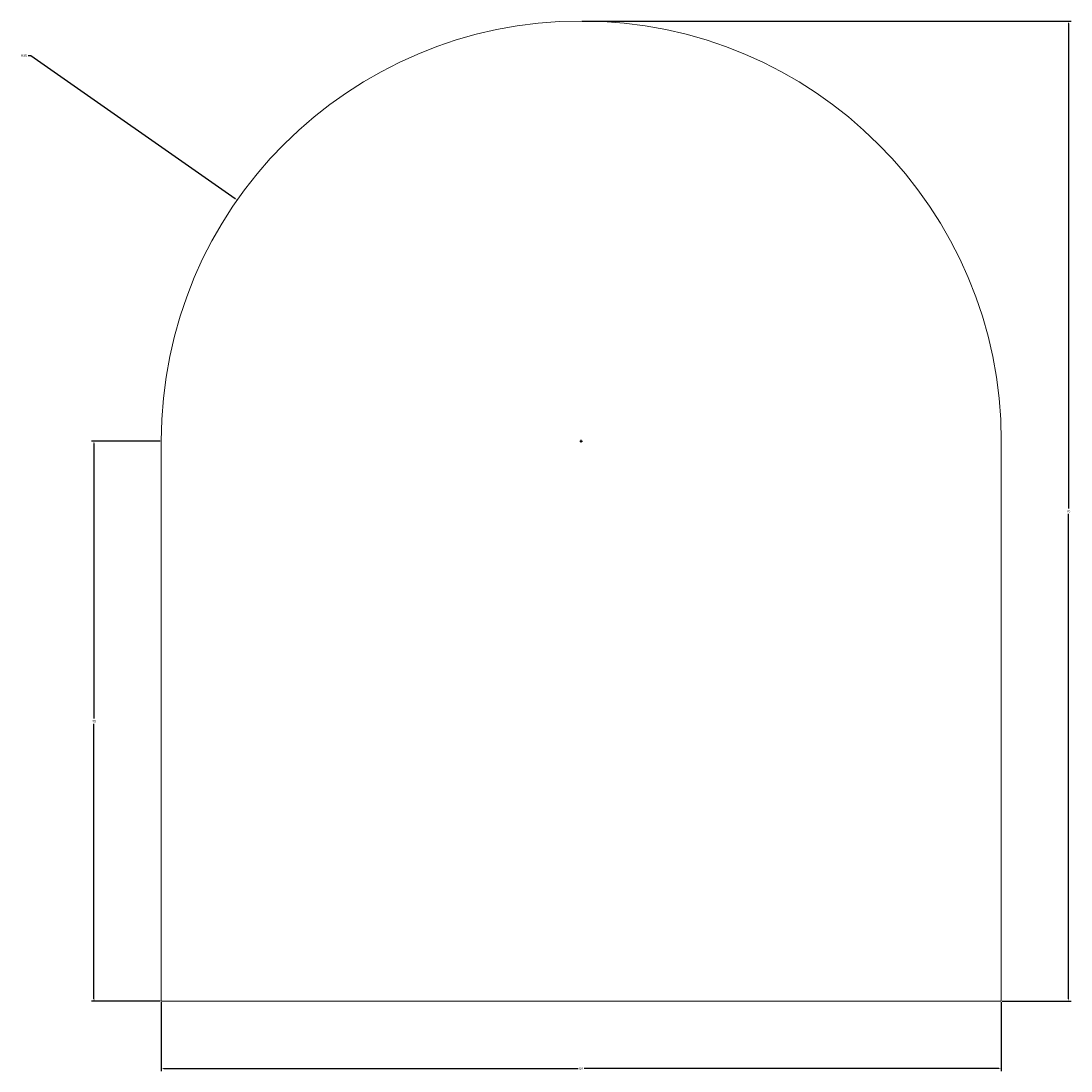
# Model space of a CAD drawing. Units: millimetres. Extents: x 0 to 390, y -312 to 42.
# Tile 2 of 3: x 207 to 282, y -312 to -237. Entities that reach past the tile are written whole.
import ezdxf

# ---------------------------------------------------------------- set-up
doc = ezdxf.new("R2010")
doc.units = ezdxf.units.MM
doc.layers.add('M-CONS', color=8, linetype='Continuous', lineweight=18)
doc.layers.add('M-DIMS', color=2, linetype='Continuous', lineweight=18)
doc.styles.get("Standard").update_dxf_attribs({"font": 'arial.ttf'})
doc.dimstyles.get("Standard").update_dxf_attribs({"dimtxt": 0.18, "dimasz": 0.18, "dimexe": 0.18, "dimexo": 0.0625, "dimgap": 0.09, "dimtad": 0, "dimtih": 1, "dimtoh": 1, "dimdec": 4, "dimzin": 0, "dimdsep": 46, "dimtxsty": 'Standard', "dimcen": 0.09, "dimadec": 0, "dimazin": 0, "dimtfac": 1, "dimtdec": 4, "dimtofl": 0, "dimtmove": 0, "dimatfit": 3, "dimfxl": 1, "dimtolj": 1, "dimtzin": 0, "dimarcsym": 0})

# ---------------------------------------------------------------- blocks, each defined once
blk = doc.blocks.new('*D1')
at = {"layer": 'Defpoints', "color": 0, "transparency": 16777216}
for p in [(216.872, -306.613), (276.872, -306.613), (276.872, -311.413)]:
    blk.add_point(p, dxfattribs=at)
at = {"layer": 'M-DIMS', "color": 0, "lineweight": -2, "transparency": 16777216}
for p, q in [((216.872, -306.675), (216.872, -311.593)), ((276.872, -306.675), (276.872, -311.593)), ((217.052, -311.413), (246.652, -311.413)), ((276.692, -311.413), (247.091, -311.413))]:
    blk.add_line(p, q, dxfattribs=at)
at = {"layer": 'M-DIMS', "color": 0, "transparency": 16777216}
for points in [[(217.052, -311.383), (217.052, -311.443), (216.872, -311.413)], [(276.692, -311.383), (276.692, -311.443), (276.872, -311.413)]]:
    blk.add_solid(points, dxfattribs=at)
at = {"layer": 'M-DIMS', "color": 0, "transparency": 16777216, "insert": (246.872, -311.413), "char_height": 0.18, "attachment_point": 5}
blk.add_mtext('\\A1;60', dxfattribs=at)
blk = doc.blocks.new('*D2')
at = {"layer": 'Defpoints', "color": 0, "transparency": 16777216}
for p in [(212.072, -266.613), (216.872, -266.613), (216.872, -306.613)]:
    blk.add_point(p, dxfattribs=at)
at = {"layer": 'M-DIMS', "color": 0, "lineweight": -2, "transparency": 16777216}
for p, q in [((216.809, -266.613), (211.892, -266.613)), ((212.072, -266.793), (212.072, -286.431)), ((212.072, -306.433), (212.072, -286.795)), ((216.809, -306.613), (211.892, -306.613))]:
    blk.add_line(p, q, dxfattribs=at)
at = {"layer": 'M-DIMS', "color": 0, "transparency": 16777216}
for points in [[(212.042, -266.793), (212.102, -266.793), (212.072, -266.613)], [(212.042, -306.433), (212.102, -306.433), (212.072, -306.613)]]:
    blk.add_solid(points, dxfattribs=at)
at = {"layer": 'M-DIMS', "color": 0, "transparency": 16777216, "insert": (212.072, -286.613), "char_height": 0.18, "attachment_point": 5}
blk.add_mtext('\\A1;40', dxfattribs=at)
blk = doc.blocks.new('*D3')
at = {"layer": 'Defpoints', "color": 0, "transparency": 16777216}
for p in [(246.872, -236.613), (281.672, -236.613), (276.872, -306.613)]:
    blk.add_point(p, dxfattribs=at)
at = {"layer": 'M-DIMS', "color": 0, "lineweight": -2, "transparency": 16777216}
for p, q in [((246.934, -236.613), (281.852, -236.613)), ((281.672, -236.793), (281.672, -271.431)), ((281.672, -306.433), (281.672, -271.795)), ((276.934, -306.613), (281.852, -306.613))]:
    blk.add_line(p, q, dxfattribs=at)
at = {"layer": 'M-DIMS', "color": 0, "transparency": 16777216}
for points in [[(281.642, -236.793), (281.702, -236.793), (281.672, -236.613)], [(281.642, -306.433), (281.702, -306.433), (281.672, -306.613)]]:
    blk.add_solid(points, dxfattribs=at)
at = {"layer": 'M-DIMS', "color": 0, "transparency": 16777216, "insert": (281.672, -271.613), "char_height": 0.18, "attachment_point": 5}
blk.add_mtext('\\A1;70', dxfattribs=at)
blk = doc.blocks.new('*D11')
at = {"layer": 'Defpoints', "color": 0, "transparency": 16777216}
for p in [(222.3, -249.4), (246.872, -266.613)]:
    blk.add_point(p, dxfattribs=at)
at = {"layer": 'M-DIMS', "color": 0, "lineweight": -2, "transparency": 16777216}
for p, q in [((207.378, -239.073), (207.558, -239.073)), ((207.558, -239.073), (222.153, -249.297)), ((246.782, -266.613), (246.962, -266.613)), ((246.872, -266.703), (246.872, -266.523))]:
    blk.add_line(p, q, dxfattribs=at)
at = {"layer": 'M-DIMS', "color": 0, "transparency": 16777216}
blk.add_solid([(222.17, -249.272), (222.136, -249.322), (222.3, -249.4)], dxfattribs=at)
at = {"layer": 'M-DIMS', "color": 0, "transparency": 16777216, "insert": (207.073, -239.073), "char_height": 0.18, "attachment_point": 5}
blk.add_mtext('\\A1;R30', dxfattribs=at)

msp = doc.modelspace()

# ---------------------------------------------------------------- linework, layer by layer
at = {"layer": 'M-CONS'}
msp.add_lwpolyline([(276.872, -266.613, 1), (216.872, -266.613), (216.872, -306.613), (276.872, -306.613)], format="xyb", close=True, dxfattribs=at)

# ---------------------------------------------------------------- dimensions: what is measured, and where the dimension line sits
at = {"layer": 'M-DIMS'}
for base, p1, p2, picture, middle in [((281.672, -236.613), (276.872, -306.613), (246.872, -236.613), '*D3', (281.672, -271.613)), ((212.072, -266.613), (216.872, -306.613), (216.872, -266.613), '*D2', (212.072, -286.613))]:
    dim = msp.add_linear_dim(base=base, p1=p1, p2=p2, angle=90, dimstyle='Standard', override={"dimdec": 0, "dimlfac": 1, "dimrnd": 0, "dimzin": 0, "dimdsep": 46, "dimlunit": 2}, dxfattribs=at)
    dim.commit()
    dim.dimension.update_dxf_attribs({"geometry": picture, "text_midpoint": middle})
dim = msp.add_radius_dim(center=(246.872, -266.613), mpoint=(222.3, -249.4), dimstyle='Standard', override={"dimdec": 0, "dimlfac": 1, "dimrnd": 0, "dimzin": 0, "dimdsep": 46, "dimlunit": 2}, dxfattribs=at)
dim.commit()
dim.dimension.update_dxf_attribs({"geometry": '*D11', "text_midpoint": (207.073, -239.073), "dimtype": 164})
dim = msp.add_linear_dim(base=(276.872, -311.413), p1=(216.872, -306.613), p2=(276.872, -306.613), dimstyle='Standard', override={"dimdec": 0, "dimlfac": 1, "dimrnd": 0, "dimzin": 0, "dimdsep": 46, "dimlunit": 2}, dxfattribs=at)
dim.commit()
dim.dimension.update_dxf_attribs({"geometry": '*D1', "text_midpoint": (246.872, -311.413)})

doc.saveas('drawing.dxf')
